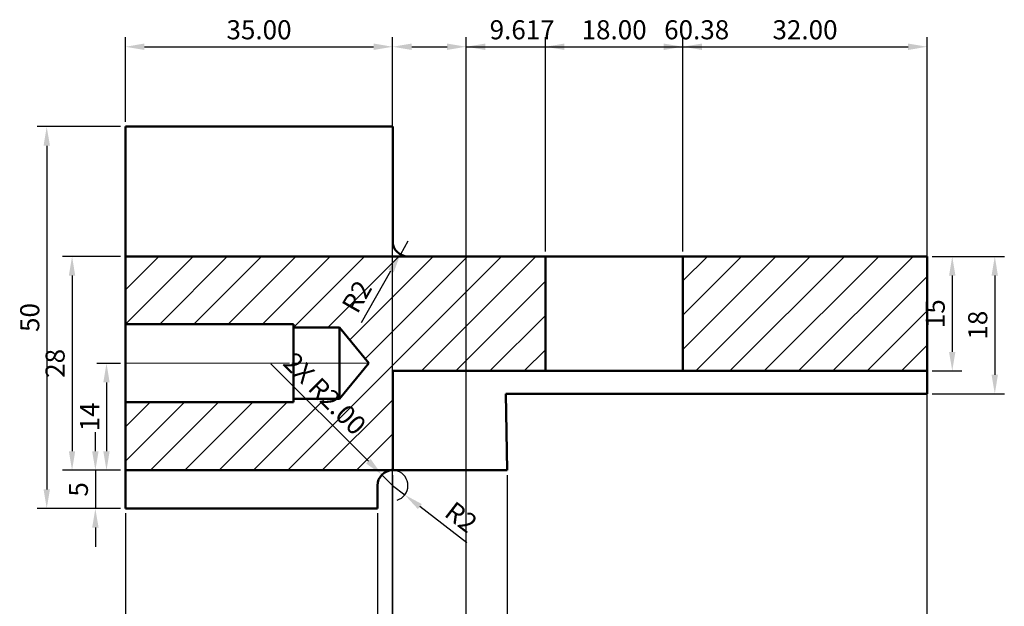
# Model space of a CAD drawing. Units: millimetres. Extents: x 2319 to 2465, y 1802 to 2026.
# Tile 2 of 2: x 2327 to 2456, y 1949 to 2026. Entities that reach past the tile are written whole.
import ezdxf

# ---------------------------------------------------------------- set-up
doc = ezdxf.new("R2010")
doc.units = ezdxf.units.MM
doc.linetypes.add('CENTER', pattern=[50.8, 31.75, -6.35, 6.35, -6.35])
for name, color, linetype, lineweight in [('M-CNTR', 1, 'CENTER', 18), ('M-DIMS', 2, 'Continuous', 25), ('M-HATC', 8, 'Continuous', 18), ('M-OUTL', 7, 'Continuous', 50)]:
    doc.layers.add(name, color=color, linetype=linetype, lineweight=lineweight)
doc.styles.get("Standard").update_dxf_attribs({"font": 'arial.ttf'})
doc.dimstyles.new('ISO-25', dxfattribs={"dimtxt": 2.5, "dimasz": 2.5, "dimexe": 1.25, "dimexo": 0.625, "dimtad": 1, "dimtxsty": 'Standard', "dimcen": 2.5, "dimadec": 0, "dimazin": 0, "dimtfac": 1, "dimtmove": 0, "dimatfit": 3, "dimfxl": 1, "dimarcsym": 0})

# ---------------------------------------------------------------- blocks, each defined once
blk = doc.blocks.new('*D1')
at = {"layer": 'Defpoints', "color": 0, "transparency": 16777216}
for p in [(2340.51, 2011.65), (2330.21, 1961.65), (2340.51, 1961.65)]:
    blk.add_point(p, dxfattribs=at)
at = {"layer": 'M-DIMS', "color": 0, "lineweight": -2, "transparency": 16777216}
for p, q in [((2339.89, 2011.65), (2328.96, 2011.65)), ((2330.21, 2009.15), (2330.21, 1964.15)), ((2339.89, 1961.65), (2328.96, 1961.65))]:
    blk.add_line(p, q, dxfattribs=at)
at = {"layer": 'M-DIMS', "color": 0, "transparency": 16777216}
for points in [[(2329.8, 2009.15), (2330.63, 2009.15), (2330.21, 2011.65)], [(2329.8, 1964.15), (2330.63, 1964.15), (2330.21, 1961.65)]]:
    blk.add_solid(points, dxfattribs=at)
at = {"layer": 'M-DIMS', "color": 0, "transparency": 16777216, "insert": (2328.31, 1986.65), "char_height": 2.5, "attachment_point": 5, "rotation": 90}
blk.add_mtext('50', dxfattribs=at)
blk = doc.blocks.new('*D2')
at = {"layer": 'Defpoints', "color": 0, "transparency": 16777216}
for p in [(2340.51, 1994.65), (2333.53, 1966.65), (2340.51, 1966.65)]:
    blk.add_point(p, dxfattribs=at)
at = {"layer": 'M-DIMS', "color": 0, "lineweight": -2, "transparency": 16777216}
for p, q in [((2339.89, 1994.65), (2332.28, 1994.65)), ((2333.53, 1992.15), (2333.53, 1969.15)), ((2339.89, 1966.65), (2332.28, 1966.65))]:
    blk.add_line(p, q, dxfattribs=at)
at = {"layer": 'M-DIMS', "color": 0, "transparency": 16777216}
for points in [[(2333.11, 1992.15), (2333.94, 1992.15), (2333.53, 1994.65)], [(2333.11, 1969.15), (2333.94, 1969.15), (2333.53, 1966.65)]]:
    blk.add_solid(points, dxfattribs=at)
at = {"layer": 'M-DIMS', "color": 0, "transparency": 16777216, "insert": (2331.63, 1980.65), "char_height": 2.5, "attachment_point": 5, "rotation": 90}
blk.add_mtext('28', dxfattribs=at)
blk = doc.blocks.new('*D3')
at = {"layer": 'Defpoints', "color": 0, "transparency": 16777216}
for p in [(2340.51, 1980.65), (2338.04, 1966.65), (2340.51, 1966.65)]:
    blk.add_point(p, dxfattribs=at)
at = {"layer": 'M-DIMS', "color": 0, "lineweight": -2, "transparency": 16777216}
for p, q in [((2339.89, 1980.65), (2336.79, 1980.65)), ((2338.04, 1978.15), (2338.04, 1969.15)), ((2339.89, 1966.65), (2336.79, 1966.65))]:
    blk.add_line(p, q, dxfattribs=at)
at = {"layer": 'M-DIMS', "color": 0, "transparency": 16777216}
for points in [[(2337.62, 1978.15), (2338.45, 1978.15), (2338.04, 1980.65)], [(2337.62, 1969.15), (2338.45, 1969.15), (2338.04, 1966.65)]]:
    blk.add_solid(points, dxfattribs=at)
at = {"layer": 'M-DIMS', "color": 0, "transparency": 16777216, "insert": (2336.16, 1973.65), "char_height": 2.5, "attachment_point": 5, "rotation": 90}
blk.add_mtext('14', dxfattribs=at)
blk = doc.blocks.new('*D4')
at = {"layer": 'Defpoints', "color": 0, "transparency": 16777216}
for p in [(2340.51, 1966.65), (2336.58, 1961.65), (2340.51, 1961.65)]:
    blk.add_point(p, dxfattribs=at)
at = {"layer": 'M-DIMS', "color": 0, "lineweight": -2, "transparency": 16777216}
for p, q in [((2336.58, 1969.15), (2336.58, 1971.65)), ((2339.89, 1966.65), (2335.33, 1966.65)), ((2336.58, 1966.65), (2336.58, 1961.65)), ((2339.89, 1961.65), (2335.33, 1961.65)), ((2336.58, 1959.15), (2336.58, 1956.65))]:
    blk.add_line(p, q, dxfattribs=at)
at = {"layer": 'M-DIMS', "color": 0, "transparency": 16777216}
for points in [[(2336.16, 1969.15), (2337, 1969.15), (2336.58, 1966.65)], [(2336.16, 1959.15), (2337, 1959.15), (2336.58, 1961.65)]]:
    blk.add_solid(points, dxfattribs=at)
at = {"layer": 'M-DIMS', "color": 0, "transparency": 16777216, "insert": (2334.68, 1964.15), "char_height": 2.5, "attachment_point": 5, "rotation": 90}
blk.add_mtext('5', dxfattribs=at)
blk = doc.blocks.new('*D5')
at = {"layer": 'Defpoints', "color": 0, "transparency": 16777216}
for p in [(2445.51, 1994.65), (2445.51, 1979.65), (2448.79, 1979.65)]:
    blk.add_point(p, dxfattribs=at)
at = {"layer": 'M-DIMS', "color": 0, "lineweight": -2, "transparency": 16777216}
for p, q in [((2446.14, 1994.65), (2450.04, 1994.65)), ((2448.79, 1992.15), (2448.79, 1982.15)), ((2446.14, 1979.65), (2450.04, 1979.65))]:
    blk.add_line(p, q, dxfattribs=at)
at = {"layer": 'M-DIMS', "color": 0, "transparency": 16777216}
for points in [[(2448.37, 1992.15), (2449.2, 1992.15), (2448.79, 1994.65)], [(2448.37, 1982.15), (2449.2, 1982.15), (2448.79, 1979.65)]]:
    blk.add_solid(points, dxfattribs=at)
at = {"layer": 'M-DIMS', "color": 0, "transparency": 16777216, "insert": (2446.88, 1987.15), "char_height": 2.5, "attachment_point": 5, "rotation": 90}
blk.add_mtext('15', dxfattribs=at)
blk = doc.blocks.new('*D6')
at = {"layer": 'Defpoints', "color": 0, "transparency": 16777216}
for p in [(2445.51, 1994.65), (2445.51, 1976.65), (2454.36, 1976.65)]:
    blk.add_point(p, dxfattribs=at)
at = {"layer": 'M-DIMS', "color": 0, "lineweight": -2, "transparency": 16777216}
for p, q in [((2446.14, 1994.65), (2455.61, 1994.65)), ((2454.36, 1992.15), (2454.36, 1979.15)), ((2446.14, 1976.65), (2455.61, 1976.65))]:
    blk.add_line(p, q, dxfattribs=at)
at = {"layer": 'M-DIMS', "color": 0, "transparency": 16777216}
for points in [[(2453.94, 1992.15), (2454.77, 1992.15), (2454.36, 1994.65)], [(2453.94, 1979.15), (2454.77, 1979.15), (2454.36, 1976.65)]]:
    blk.add_solid(points, dxfattribs=at)
at = {"layer": 'M-DIMS', "color": 0, "transparency": 16777216, "insert": (2452.45, 1985.65), "char_height": 2.5, "attachment_point": 5, "rotation": 90}
blk.add_mtext('18', dxfattribs=at)
blk = doc.blocks.new('*D7')
at = {"layer": 'Defpoints', "color": 0, "transparency": 16777216}
for p in [(2377.51, 1996.65), (2376.52, 1994.91)]:
    blk.add_point(p, dxfattribs=at)
at = {"layer": 'M-DIMS', "color": 0, "lineweight": -2, "transparency": 16777216}
for p, q in [((2377.51, 1996.65), (2376.52, 1994.91)), ((2371.42, 1986.02), (2375.28, 1992.75))]:
    blk.add_line(p, q, dxfattribs=at)
at = {"layer": 'M-DIMS', "color": 0, "transparency": 16777216}
blk.add_solid([(2374.92, 1992.95), (2375.64, 1992.54), (2376.52, 1994.91)], dxfattribs=at)
at = {"layer": 'M-DIMS', "color": 0, "transparency": 16777216, "insert": (2371.1, 1989.23), "char_height": 2.5, "attachment_point": 5, "rotation": 60.1907}
blk.add_mtext('R2', dxfattribs=at)
blk = doc.blocks.new('*D8')
at = {"layer": 'Defpoints', "color": 0, "transparency": 16777216}
for p in [(2375.51, 1964.65), (2377.1, 1963.43)]:
    blk.add_point(p, dxfattribs=at)
at = {"layer": 'M-DIMS', "color": 0, "lineweight": -2, "transparency": 16777216}
for p, q in [((2375.51, 1964.65), (2377.1, 1963.43)), ((2385.22, 1957.16), (2379.08, 1961.9))]:
    blk.add_line(p, q, dxfattribs=at)
blk.add_arc((2375.51, 1964.65), 2, 286.5453, 72.0951, dxfattribs=at)
at = {"layer": 'M-DIMS', "color": 0, "transparency": 16777216}
blk.add_solid([(2379.33, 1962.23), (2378.82, 1961.57), (2377.1, 1963.43)], dxfattribs=at)
at = {"layer": 'M-DIMS', "color": 0, "transparency": 16777216, "insert": (2384.29, 1960.26), "char_height": 2.5, "attachment_point": 5, "rotation": 322.3551}
blk.add_mtext('R2', dxfattribs=at)
blk = doc.blocks.new('*D32')
at = {"layer": 'Defpoints', "color": 0, "transparency": 16777216}
for p in [(2445.51, 2022.1), (2385.13, 1912.15), (2445.51, 1912.15)]:
    blk.add_point(p, dxfattribs=at)
at = {"layer": 'M-DIMS', "color": 0, "lineweight": -2, "transparency": 16777216}
for p, q in [((2385.13, 1912.77), (2385.13, 2023.35)), ((2445.51, 1912.77), (2445.51, 2023.35)), ((2387.63, 2022.1), (2443.01, 2022.1))]:
    blk.add_line(p, q, dxfattribs=at)
at = {"layer": 'M-DIMS', "color": 0, "transparency": 16777216}
for points in [[(2387.63, 2022.52), (2387.63, 2021.68), (2385.13, 2022.1)], [(2443.01, 2022.52), (2443.01, 2021.68), (2445.51, 2022.1)]]:
    blk.add_solid(points, dxfattribs=at)
at = {"layer": 'M-DIMS', "color": 0, "transparency": 16777216, "insert": (2415.32, 2024), "char_height": 2.5, "attachment_point": 5}
blk.add_mtext('60.38', dxfattribs=at)
blk = doc.blocks.new('*D33')
at = {"layer": 'Defpoints', "color": 0, "transparency": 16777216}
for p in [(2375.51, 2022.1), (2340.51, 2011.65), (2375.51, 2011.65)]:
    blk.add_point(p, dxfattribs=at)
at = {"layer": 'M-DIMS', "color": 0, "lineweight": -2, "transparency": 16777216}
for p, q in [((2340.51, 2012.28), (2340.51, 2023.35)), ((2375.51, 2012.28), (2375.51, 2023.35)), ((2343.01, 2022.1), (2373.01, 2022.1))]:
    blk.add_line(p, q, dxfattribs=at)
at = {"layer": 'M-DIMS', "color": 0, "transparency": 16777216}
for points in [[(2343.01, 2022.52), (2343.01, 2021.68), (2340.51, 2022.1)], [(2373.01, 2022.52), (2373.01, 2021.68), (2375.51, 2022.1)]]:
    blk.add_solid(points, dxfattribs=at)
at = {"layer": 'M-DIMS', "color": 0, "transparency": 16777216, "insert": (2358.01, 2024), "char_height": 2.5, "attachment_point": 5}
blk.add_mtext('35.00', dxfattribs=at)
blk = doc.blocks.new('*D34')
at = {"layer": 'Defpoints', "color": 0, "transparency": 16777216}
for p in [(2413.51, 2022.1), (2395.51, 1994.65), (2413.51, 1994.65)]:
    blk.add_point(p, dxfattribs=at)
at = {"layer": 'M-DIMS', "color": 0, "lineweight": -2, "transparency": 16777216}
for p, q in [((2395.51, 1995.28), (2395.51, 2023.35)), ((2413.51, 1995.28), (2413.51, 2023.35)), ((2398.01, 2022.1), (2411.01, 2022.1))]:
    blk.add_line(p, q, dxfattribs=at)
at = {"layer": 'M-DIMS', "color": 0, "transparency": 16777216}
for points in [[(2398.01, 2022.52), (2398.01, 2021.68), (2395.51, 2022.1)], [(2411.01, 2022.52), (2411.01, 2021.68), (2413.51, 2022.1)]]:
    blk.add_solid(points, dxfattribs=at)
at = {"layer": 'M-DIMS', "color": 0, "transparency": 16777216, "insert": (2404.51, 2024), "char_height": 2.5, "attachment_point": 5}
blk.add_mtext('18.00', dxfattribs=at)
blk = doc.blocks.new('*D35')
at = {"layer": 'Defpoints', "color": 0, "transparency": 16777216}
for p in [(2445.51, 2022.1), (2413.51, 1994.65), (2445.51, 1994.65)]:
    blk.add_point(p, dxfattribs=at)
at = {"layer": 'M-DIMS', "color": 0, "lineweight": -2, "transparency": 16777216}
for p, q in [((2413.51, 1995.28), (2413.51, 2023.35)), ((2445.51, 1995.28), (2445.51, 2023.35)), ((2416.01, 2022.1), (2443.01, 2022.1))]:
    blk.add_line(p, q, dxfattribs=at)
at = {"layer": 'M-DIMS', "color": 0, "transparency": 16777216}
for points in [[(2416.01, 2022.52), (2416.01, 2021.68), (2413.51, 2022.1)], [(2443.01, 2022.52), (2443.01, 2021.68), (2445.51, 2022.1)]]:
    blk.add_solid(points, dxfattribs=at)
at = {"layer": 'M-DIMS', "color": 0, "transparency": 16777216, "insert": (2429.51, 2024), "char_height": 2.5, "attachment_point": 5}
blk.add_mtext('32.00', dxfattribs=at)
blk = doc.blocks.new('*D36')
at = {"layer": 'Defpoints', "color": 0, "transparency": 16777216}
for p in [(2340.51, 1961.65), (2373.51, 1961.65), (2373.51, 1803.7)]:
    blk.add_point(p, dxfattribs=at)
at = {"layer": 'M-DIMS', "color": 0, "lineweight": -2, "transparency": 16777216}
for p, q in [((2340.51, 1961.03), (2340.51, 1802.45)), ((2373.51, 1961.03), (2373.51, 1802.45)), ((2343.01, 1803.7), (2371.01, 1803.7))]:
    blk.add_line(p, q, dxfattribs=at)
at = {"layer": 'M-DIMS', "color": 0, "transparency": 16777216}
for points in [[(2343.01, 1804.12), (2343.01, 1803.28), (2340.51, 1803.7)], [(2371.01, 1804.12), (2371.01, 1803.28), (2373.51, 1803.7)]]:
    blk.add_solid(points, dxfattribs=at)
at = {"layer": 'M-DIMS', "color": 0, "transparency": 16777216, "insert": (2357.01, 1805.6), "char_height": 2.5, "attachment_point": 5}
blk.add_mtext('33.00', dxfattribs=at)
blk = doc.blocks.new('*D37')
at = {"layer": 'Defpoints', "color": 0, "transparency": 16777216}
for p in [(2375.51, 1966.65), (2390.51, 1966.65), (2390.51, 1803.7)]:
    blk.add_point(p, dxfattribs=at)
at = {"layer": 'M-DIMS', "color": 0, "lineweight": -2, "transparency": 16777216}
for p, q in [((2375.51, 1966.03), (2375.51, 1802.45)), ((2390.51, 1966.03), (2390.51, 1802.45)), ((2378.01, 1803.7), (2388.01, 1803.7))]:
    blk.add_line(p, q, dxfattribs=at)
at = {"layer": 'M-DIMS', "color": 0, "transparency": 16777216}
for points in [[(2378.01, 1804.12), (2378.01, 1803.28), (2375.51, 1803.7)], [(2388.01, 1804.12), (2388.01, 1803.28), (2390.51, 1803.7)]]:
    blk.add_solid(points, dxfattribs=at)
at = {"layer": 'M-DIMS', "color": 0, "transparency": 16777216, "insert": (2383.01, 1805.6), "char_height": 2.5, "attachment_point": 5}
blk.add_mtext('15.00', dxfattribs=at)
blk = doc.blocks.new('*D38')
at = {"layer": 'Defpoints', "color": 0, "transparency": 16777216}
for p in [(2385.13, 2022.1), (2385.13, 1912.15), (2375.51, 1906.15)]:
    blk.add_point(p, dxfattribs=at)
at = {"layer": 'M-DIMS', "color": 0, "lineweight": -2, "transparency": 16777216}
for p, q in [((2375.51, 1906.77), (2375.51, 2023.35)), ((2385.13, 1912.77), (2385.13, 2023.35)), ((2378.01, 2022.1), (2382.63, 2022.1)), ((2385.13, 2022.1), (2397.32, 2022.1))]:
    blk.add_line(p, q, dxfattribs=at)
at = {"layer": 'M-DIMS', "color": 0, "transparency": 16777216}
for points in [[(2378.01, 2022.52), (2378.01, 2021.68), (2375.51, 2022.1)], [(2382.63, 2022.52), (2382.63, 2021.68), (2385.13, 2022.1)]]:
    blk.add_solid(points, dxfattribs=at)
at = {"layer": 'M-DIMS', "color": 0, "transparency": 16777216, "insert": (2392.47, 2024), "char_height": 2.5, "attachment_point": 5}
blk.add_mtext('9.617', dxfattribs=at)
blk = doc.blocks.new('*D43')
at = {"layer": 'Defpoints', "color": 0, "transparency": 16777216}
for p in [(2374.1, 1966.06), (2375.51, 1964.65)]:
    blk.add_point(p, dxfattribs=at)
at = {"layer": 'M-DIMS', "color": 0, "lineweight": -2, "transparency": 16777216}
for p, q in [((2359.57, 1980.59), (2372.33, 1967.83)), ((2375.51, 1964.65), (2374.1, 1966.06))]:
    blk.add_line(p, q, dxfattribs=at)
at = {"layer": 'M-DIMS', "color": 0, "transparency": 16777216}
blk.add_solid([(2372.63, 1968.13), (2372.04, 1967.54), (2374.1, 1966.06)], dxfattribs=at)
at = {"layer": 'M-DIMS', "color": 0, "transparency": 16777216, "insert": (2366.41, 1976.44), "char_height": 2.5, "attachment_point": 5, "rotation": 315.0048}
blk.add_mtext('2X R2.00', dxfattribs=at)

msp = doc.modelspace()

# ---------------------------------------------------------------- hatches: boundary and pattern name
at = {"layer": 'M-HATC'}
h = msp.add_hatch(dxfattribs=at)
h.set_pattern_fill('ANSI31', color=256)
h.paths.add_polyline_path([(2395.514, 1994.6502), (2340.514, 1994.6502), (2340.514, 1985.7502), (2362.514, 1985.7502), (2362.514, 1985.3128), (2368.5282, 1985.3128), (2372.3842, 1980.6502), (2368.5282, 1975.9902), (2362.514, 1975.9902), (2362.514, 1975.5502), (2340.514, 1975.5502), (2340.514, 1966.6502), (2375.514, 1966.6502), (2375.514, 1979.6502), (2395.514, 1979.6502)])
h.paths.add_polyline_path([(2445.514, 1994.6502), (2413.514, 1994.6502), (2413.514, 1979.6502), (2445.514, 1979.6502)])

# ---------------------------------------------------------------- linework, layer by layer
at = {"layer": 'M-CNTR'}
for p, q in [((2340.514, 1980.6633), (2362.0007, 1980.6633)), ((2362.292, 1980.6633), (2368.5282, 1980.6633)), ((2368.5282, 1980.6633), (2372.3842, 1980.6633))]:
    msp.add_line(p, q, dxfattribs=at)
at = {"layer": 'M-OUTL'}
for p, q in [((2340.514, 1961.6502), (2340.514, 2011.6502)), ((2340.514, 2011.6502), (2375.514, 2011.6502)), ((2375.514, 2011.6502), (2375.514, 1996.6502)), ((2340.514, 1994.6502), (2445.514, 1994.6502)), ((2340.514, 1976.6502), (2340.514, 1994.6502)), ((2340.514, 1994.6502), (2340.514, 1966.6502)), ((2395.514, 1979.6502), (2395.514, 1994.6502)), ((2413.514, 1987.1502), (2413.514, 1994.6502)), ((2413.514, 1994.6502), (2413.514, 1979.6502)), ((2445.514, 1994.6502), (2445.514, 1979.6502)), ((2340.514, 1985.7633), (2362.514, 1985.7633)), ((2340.514, 1980.6502), (2340.514, 1985.7502)), ((2362.514, 1985.7633), (2362.514, 1975.5633)), ((2362.514, 1985.7502), (2362.514, 1975.5502)), ((2362.514, 1985.326), (2368.5282, 1985.326)), ((2362.514, 1980.6502), (2362.514, 1985.3128)), ((2368.5282, 1985.326), (2368.5282, 1976.0033)), ((2372.3842, 1980.6633), (2368.5282, 1985.326)), ((2340.514, 1966.6502), (2340.514, 1980.6502)), ((2340.514, 1966.6502), (2340.514, 1980.6502)), ((2362.514, 1980.6502), (2362.514, 1975.9902)), ((2368.5282, 1976.0033), (2372.3842, 1980.6633)), ((2445.514, 1979.6502), (2375.514, 1979.6502)), ((2375.514, 1979.6502), (2375.514, 1976.6502)), ((2375.514, 1966.6502), (2375.514, 1979.6502)), ((2413.514, 1979.6502), (2395.514, 1979.6502)), ((2445.514, 1979.6502), (2445.514, 1976.6502)), ((2340.514, 1976.6502), (2340.514, 1971.6502)), ((2445.514, 1976.6502), (2390.3487, 1976.6502)), ((2390.3487, 1976.6502), (2390.514, 1966.6502)), ((2362.514, 1975.5633), (2340.514, 1975.5633)), ((2362.514, 1976.0033), (2368.5282, 1976.0033)), ((2340.514, 1966.6502), (2375.514, 1966.6502)), ((2340.514, 1966.6502), (2340.514, 1961.6502)), ((2375.514, 1966.6502), (2370.514, 1966.6502)), ((2375.514, 1966.6502), (2373.514, 1966.6502)), ((2375.514, 1966.6502), (2373.514, 1966.6502)), ((2375.514, 1966.6502), (2390.514, 1966.6502)), ((2373.514, 1964.6502), (2373.514, 1961.6502)), ((2340.514, 1961.6502), (2373.514, 1961.6502))]:
    msp.add_line(p, q, dxfattribs=at)
for centre, start, end in [((2377.514, 1996.6502), 180, 270), ((2375.514, 1964.6502), 90, 180)]:
    msp.add_arc(centre, 2, start, end, dxfattribs=at)

# ---------------------------------------------------------------- dimensions: what is measured, and where the dimension line sits
at = {"layer": 'M-DIMS'}
for base, p1, p2, override, picture, middle in [((2375.514, 2022.1002), (2340.514, 2011.6502), (2375.514, 2011.6502), {"dimdec": 2, "dimlfac": 1, "dimrnd": 0, "dimzin": 0, "dimdsep": 46, "dimlunit": 2}, '*D33', (2358.014, 2024.0025)), ((2385.1309, 2022.1002), (2375.514, 1906.1497), (2385.1309, 1912.1497), {"dimdec": 3, "dimlfac": 1, "dimrnd": 0, "dimzin": 0, "dimdsep": 46, "dimlunit": 2}, '*D38', (2392.474, 2024.0017)), ((2445.514, 2022.1002), (2385.1309, 1912.1497), (2445.514, 1912.1497), {"dimdec": 2, "dimlfac": 1, "dimrnd": 0, "dimzin": 0, "dimdsep": 46, "dimlunit": 2}, '*D32', (2415.3224, 2024.0025)), ((2413.514, 2022.1002), (2395.514, 1994.6502), (2413.514, 1994.6502), {"dimdec": 2, "dimlfac": 1, "dimrnd": 0, "dimzin": 0, "dimdsep": 46, "dimlunit": 2}, '*D34', (2404.514, 2024.0017)), ((2445.514, 2022.1002), (2413.514, 1994.6502), (2445.514, 1994.6502), {"dimdec": 2, "dimlfac": 1, "dimrnd": 0, "dimzin": 0, "dimdsep": 46, "dimlunit": 2}, '*D35', (2429.514, 2024.0025)), ((2390.514, 1803.6997), (2375.514, 1966.6502), (2390.514, 1966.6502), {"dimdec": 2, "dimlfac": 1, "dimrnd": 0, "dimzin": 0, "dimdsep": 46, "dimlunit": 2}, '*D37', (2383.014, 1805.6011)), ((2373.514, 1803.6997), (2340.514, 1961.6502), (2373.514, 1961.6502), {"dimdec": 2, "dimlfac": 1, "dimrnd": 0, "dimzin": 0, "dimdsep": 46, "dimlunit": 2}, '*D36', (2357.014, 1805.602))]:
    dim = msp.add_linear_dim(base=base, p1=p1, p2=p2, dimstyle='ISO-25', override=override, dxfattribs=at)
    dim.commit()
    dim.dimension.update_dxf_attribs({"geometry": picture, "text_midpoint": middle})
for base, p1, p2, picture, middle in [((2330.2124, 1961.6502), (2340.514, 2011.6502), (2340.514, 1961.6502), '*D1', (2328.3109, 1986.6502)), ((2333.5282, 1966.6502), (2340.514, 1994.6502), (2340.514, 1966.6502), '*D2', (2331.6267, 1980.6502)), ((2448.785, 1979.6502), (2445.514, 1994.6502), (2445.514, 1979.6502), '*D5', (2446.8836, 1987.1502)), ((2454.3556, 1976.6502), (2445.514, 1994.6502), (2445.514, 1976.6502), '*D6', (2452.4541, 1985.6502)), ((2338.0377, 1966.6502), (2340.514, 1980.6502), (2340.514, 1966.6502), '*D3', (2336.1575, 1973.6502)), ((2336.5787, 1961.6502), (2340.514, 1966.6502), (2340.514, 1961.6502), '*D4', (2334.6824, 1964.1502))]:
    dim = msp.add_linear_dim(base=base, p1=p1, p2=p2, angle=90, dimstyle='ISO-25', override={"dimclrd": 0, "dimclre": 0, "dimclrt": 0}, dxfattribs=at)
    dim.commit()
    dim.dimension.update_dxf_attribs({"geometry": picture, "text_midpoint": middle})
for center, mpoint, picture, middle in [((2377.514, 1996.6502), (2376.5198, 1994.9149), '*D7', (2371.0965, 1989.2309)), ((2375.514, 1964.6502), (2377.0976, 1963.4287), '*D8', (2384.2858, 1960.2585))]:
    dim = msp.add_radius_dim(center=center, mpoint=mpoint, dimstyle='ISO-25', override={"dimclrd": 0, "dimclre": 0, "dimclrt": 0}, dxfattribs=at)
    dim.commit()
    dim.dimension.update_dxf_attribs({"geometry": picture, "text_midpoint": middle})
dim = msp.add_radius_dim(center=(2375.514, 1964.6502), mpoint=(2374.0997, 1966.0643), text='2X <>', dimstyle='ISO-25', override={"dimdec": 2, "dimlfac": 1, "dimrnd": 0, "dimzin": 0, "dimdsep": 46, "dimlunit": 2}, dxfattribs=at)
dim.commit()
dim.dimension.update_dxf_attribs({"geometry": '*D43', "text_midpoint": (2366.4128, 1976.4387)})

doc.saveas('drawing.dxf')
